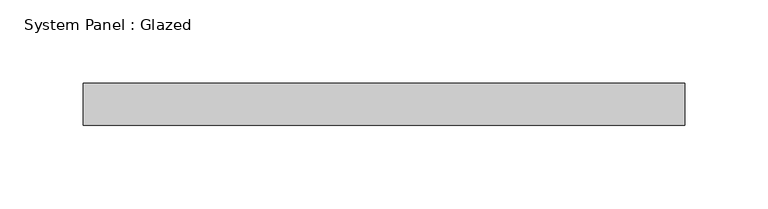
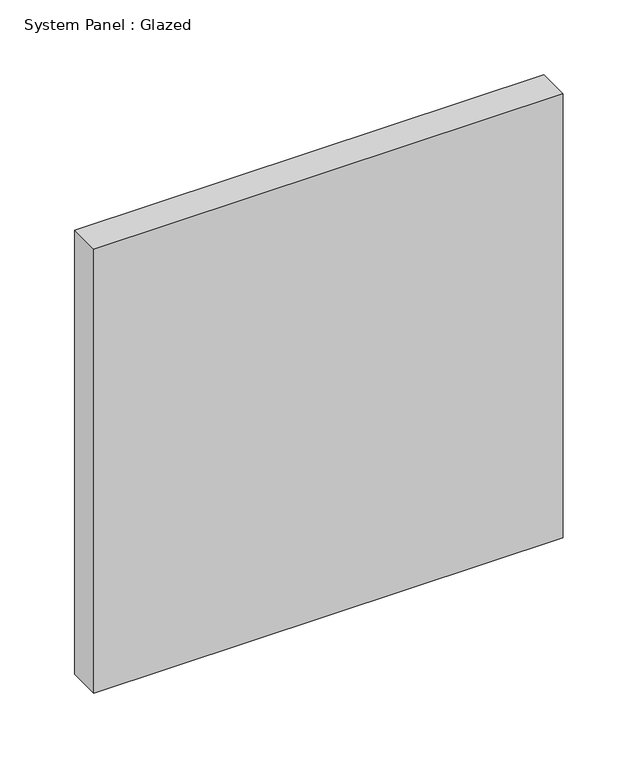
"""IFC4 building model written with IfcOpenShell, lengths in millimetres: plate geometry, System Panel : Glazed."""

from ifc_helpers import new_model, si_unit, origin, origin_with_axes, place, context, project, spatial, polyline, outline, extrude, source, transform, mapped, element, save


def system_panel_glazed_235599b7(model_context):
    return source(origin(), model_context, "Body", "SweptSolid", [
        extrude(outline(polyline([(180.975, 19.05), (-180.975, 19.05), (-180.975, 44.45), (180.975, 44.45), (180.975, 19.05)])), origin_with_axes(), (0.0, 0.0, 1.0), 361.95),
    ])


if __name__ == "__main__":
    model = new_model("IFC4")
    model_context = context("Model", 3, world=origin())
    ifc_project = project(units=[si_unit("LENGTHUNIT", "METRE", prefix="MILLI")], contexts=[model_context])
    site = spatial("IfcSite", under=ifc_project)
    building = spatial("IfcBuilding", under=site)
    placement = place(None, origin())
    system_panel_glazed_shape = system_panel_glazed_235599b7(model_context)
    element("IfcPlate", 1, ObjectType="System Panel : Glazed", at=placement, inside=building, context=model_context, shape_type="MappedRepresentation", body=[
        mapped(system_panel_glazed_shape, transform((0.0, 0.0, 0.0), x_axis=(1.0, 0.0, 0.0), y_axis=(0.0, 1.0, 0.0), z_axis=(0.0, 0.0, 1.0))),
    ])
    save(model, "model.ifc")

# Revit data of these elements
# Type "System Panel : Glazed"
#   Construction Type Id = "GSP4R"
#   Analytic Construction = "1/8 in Pilkington single glazing"
#   Visual Light Transmittance = 0.9
#   Solar Heat Gain Coefficient = 0.86
#   Heat Transfer Coefficient (U) = 1.18115 BTU/(h·ft²·°F)
#   Define Thermal Properties by = 1
# Element 1 (IfcPlate, "System Panel : Glazed")
#   Materials on its faces: "Glass"
# Materials
#   "Glass": class "Glass", colour RGB 0 128 192, transparency 0.75, Description = "Soda Lime Glass", Cost = 0
